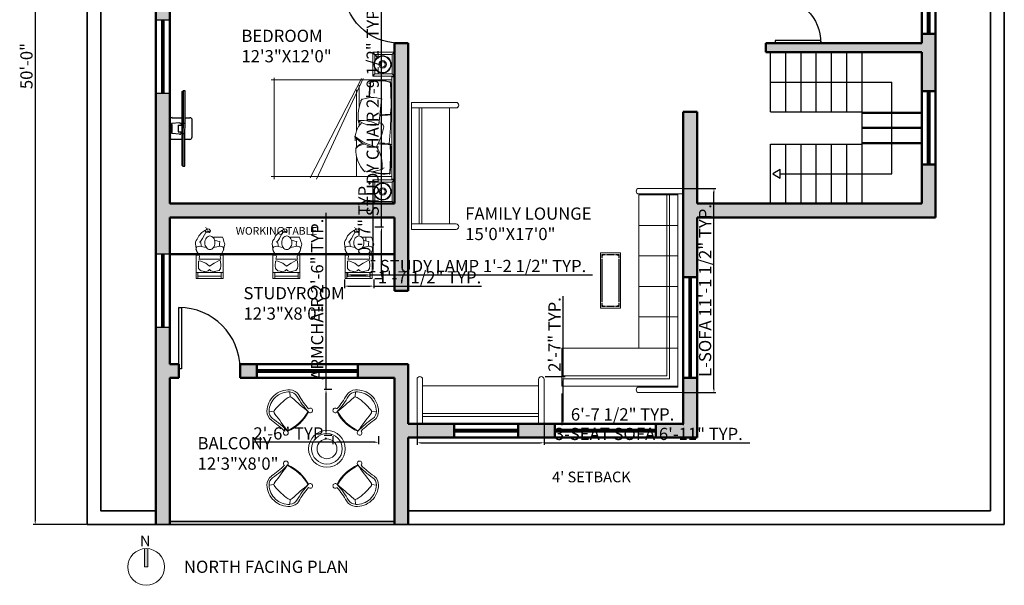
# Model space of a CAD drawing. Units: inches. Extents: x 2442 to 3851, y 589 to 2836.
# Tile 11 of 22: x 3165 to 3809, y 1362 to 1732. Entities that reach past the tile are written whole.
import ezdxf

# ---------------------------------------------------------------- set-up
doc = ezdxf.new("R2010")
doc.units = ezdxf.units.IN
for name, color, linetype, lineweight in [('0.10', 252, 'Continuous', 9), ('0.15', 34, 'Continuous', 15), ('A-ANNO-DIMS', 2, 'Continuous', 18), ('A-ANNO-SYMB', 1, 'Continuous', 18), ('A-ANNO-TEXT', 7, 'Continuous', 18), ('A-AREA-IDEN', 7, 'Continuous', 18), ('A-DOOR', 4, 'Continuous', 25), ('A-FLOR-STRS', 3, 'Continuous', 25), ('A-FURN', 8, 'Continuous', 18), ('A-GLAZ', 1, 'Continuous', 25), ('A-WALL', 7, 'Continuous', 50), ('A-WALL-PATT', 8, 'Continuous', 13), ('C-PROP', 7, 'Continuous', 35)]:
    doc.layers.add(name, color=color, linetype=linetype, lineweight=lineweight)
doc.layers.add('window', color=130, linetype='Continuous')
doc.styles.get("Standard").update_dxf_attribs({"font": 'arial.ttf'})
doc.dimstyles.new('ISO-25', dxfattribs={"dimtxt": 8, "dimasz": 2.5, "dimexe": 1.25, "dimexo": 0.625, "dimtad": 1, "dimlunit": 3, "dimtxsty": 'Standard', "dimcen": 2.5, "dimadec": 0, "dimazin": 0, "dimtfac": 1, "dimtmove": 0, "dimatfit": 3, "dimfxl": 1, "dimarcsym": 0})

# ---------------------------------------------------------------- blocks, each defined once
blk = doc.blocks.new('*U22')
for p, q in [((0, 0), (0, -6)), ((40, 0), (40, -6))]:
    blk.add_line(p, q)
blk.add_lwpolyline([(0, 0), (0, 40), (1.75, 40), (1.75, 0)], close=True)
blk.add_arc((0, 0), 40, 0, 90)
blk = doc.blocks.new('*U23')
for p, q in [((0, 0), (0, -6)), ((36, 0), (36, -6))]:
    blk.add_line(p, q)
blk.add_lwpolyline([(0, 0), (0, 36), (1.75, 36), (1.75, 0)], close=True)
blk.add_arc((0, 0), 36, 0, 90)
blk = doc.blocks.new('*U24')
for p, q in [((0, 0), (0, -6)), ((30, 0), (30, -6))]:
    blk.add_line(p, q)
blk.add_lwpolyline([(0, 0), (0, 30), (1.75, 30), (1.75, 0)], close=True)
blk.add_arc((0, 0), 30, 0, 90)
blk = doc.blocks.new('camita')
at = {"layer": '0.10'}
for p, q in [((-0.85, -0.045), (0.85, -0.045)), ((-0.805, -0.045), (-0.805, -2.048)), ((0.805, -0.045), (0.805, -2.048)), ((-0.827, -0.521), (0.846, -1.293)), ((-0.827, -0.548), (0.824, -1.399)), ((-0.716, -0.585), (-0.355, -0.585)), ((-0.638, -0.63), (0.043, -0.63)), ((-0.114, -0.585), (-0.049, -0.585)), ((0.175, -0.63), (0.318, -0.63)), ((0.474, -0.63), (0.805, -0.63)), ((-0.835, -2), (0.846, -2))]:
    blk.add_line(p, q, dxfattribs=at)
blk.add_lwpolyline([(-0.85, -0.041), (0.85, -0.041), (0.85, 0), (-0.85, 0)], close=True, dxfattribs=at)
for centre, radius, start, end in [((-0.457, -0.236), 0.344, 147.51, 213.8336), ((-0.2, -0.227), 0.586, 163.9263, 197.1409), ((-0.364, -5.846), 5.791, 83.8073, 94.1211), ((-0.51, -1.723), 1.678, 80.1255, 98.6619), ((2.353, -0.053), 2.58, 180.1063, 184.3854), ((-1.544, -0.245), 1.333, 359.9394, 7.5533), ((1.581, -0.289), 1.335, 170.3802, 178.9914), ((-1.44, -0.061), 1.712, 352.9291, 0.3959), ((0.452, -3.067), 3, 83.9026, 93.6759), ((0.486, -1.629), 1.578, 80.1602, 98.06), ((0.029, -0.138), 0.726, 342.5841, 6.0048), ((0.133, -0.17), 0.631, 339.923, 8.7433), ((-0.054, -0.363), 0.454, 159.3026, 206.5026), ((-1.33, -9.675), 9.499, 82.2708, 84.9399), ((0.458, -0.545), 0.584, 151.0456, 184.1497), ((-0.534, -0.339), 0.487, 327.2644, 9.0473), ((-0.007, -0.258), 0.0828, 100.018, 179.736), ((-0.293, -1.438), 1.29, 61.9749, 77.8435), ((-0.199, -0.274), 0.516, 310.7395, 359.0576), ((-0.567, -0.087), 0.906, 321.6953, 346.4626), ((0.627, -0.752), 0.551, 82.9691, 124.6739), ((0.32, -0.394), 0.404, 341.4524, 33.4512), ((-1.867, -14.986), 14.632, 84.6597, 85.7516), ((-0.46, 1.486), 1.909, 260.953, 268.6517), ((-0.2, 0.064), 0.667, 244.7809, 279.0606), ((0.179, -0.272), 0.383, 224.5284, 275.2229), ((0.438, -0.483), 0.19, 193.6849, 236.7035), ((0.571, -0.432), 0.315, 192.9388, 221.9636), ((0.361, -0.133), 0.51, 267.2589, 315.2997)]:
    blk.add_arc(centre, radius, start, end, dxfattribs=at)
blk = doc.blocks.new('VELADOR')
at = {"layer": '0.15'}
for p, q in [((-0.248, 0), (-0.203, -0.045)), ((0.248, 0), (0.202, -0.045)), ((-0.203, -0.405), (-0.248, -0.45)), ((0.248, -0.45), (0.202, -0.405))]:
    blk.add_line(p, q, dxfattribs=at)
blk.add_lwpolyline([(-0.248, 0), (-0.248, -0.45), (0.248, -0.45), (0.248, 0)], close=True, dxfattribs=at)
blk.add_lwpolyline([(0.092, -0.405), (0.202, -0.405), (0.202, -0.045), (-0.203, -0.045), (-0.203, -0.405), (-0.082, -0.405)], dxfattribs=at)
for radius in [0.18, 0.169, 0.0788, 0.0563]:
    blk.add_circle((0.005, -0.247), radius, dxfattribs=at)
blk = doc.blocks.new('TABLE-30A')
at = {"color": 0, "linetype": 'ByBlock'}
for p, q in [((0, 0), (0, 0.55)), ((0, 0.55), (1.5, 0.55)), ((1.5, 0.55), (1.5, 0)), ((0.051, 0.508), (0.042, 0.499)), ((0.042, 0.499), (0.042, 0.478)), ((0.042, 0.478), (0.072, 0.478)), ((0.042, 0.478), (0.042, 0.41)), ((0.042, 0.169), (0.042, 0.381)), ((0.072, 0.508), (0.051, 0.508)), ((0.051, 0.478), (0.051, 0.41)), ((0.051, 0.169), (0.051, 0.381)), ((0.072, 0.478), (0.072, 0.508)), ((0.072, 0.508), (0.14, 0.508)), ((0.072, 0.499), (0.14, 0.499)), ((1.331, 0.508), (0.169, 0.508)), ((1.331, 0.499), (0.169, 0.499)), ((1.428, 0.508), (1.36, 0.508)), ((1.428, 0.499), (1.36, 0.499)), ((1.428, 0.508), (1.428, 0.478)), ((1.449, 0.508), (1.428, 0.508)), ((1.428, 0.478), (1.458, 0.478)), ((1.458, 0.499), (1.449, 0.508)), ((1.449, 0.478), (1.449, 0.41)), ((1.449, 0.381), (1.449, 0.169)), ((1.458, 0.478), (1.458, 0.499)), ((1.458, 0.478), (1.458, 0.41)), ((1.458, 0.381), (1.458, 0.169)), ((1.5, 0), (0, 0)), ((0.042, 0.072), (0.042, 0.14)), ((0.042, 0.072), (0.042, 0.051)), ((0.072, 0.072), (0.042, 0.072)), ((0.042, 0.051), (0.051, 0.042)), ((0.051, 0.072), (0.051, 0.14)), ((0.051, 0.042), (0.072, 0.042)), ((0.072, 0.042), (0.072, 0.072)), ((0.072, 0.051), (0.14, 0.051)), ((0.072, 0.042), (0.14, 0.042)), ((0.169, 0.051), (1.331, 0.051)), ((0.169, 0.042), (1.331, 0.042)), ((1.428, 0.051), (1.36, 0.051)), ((1.428, 0.042), (1.36, 0.042)), ((1.428, 0.072), (1.428, 0.042)), ((1.458, 0.072), (1.428, 0.072)), ((1.428, 0.042), (1.449, 0.042)), ((1.449, 0.072), (1.449, 0.14)), ((1.449, 0.042), (1.458, 0.051)), ((1.458, 0.072), (1.458, 0.14)), ((1.458, 0.051), (1.458, 0.072))]:
    blk.add_line(p, q, dxfattribs=at)
blk = doc.blocks.new('TV')
at = {"color": 0}
for p, q in [((3967.27, 1784.85), (3967.05, 1784.65)), ((3967.76, 1763.68), (3967.54, 1763.86))]:
    blk.add_line(p, q, dxfattribs=at)
at = {"layer": 'window'}
for p, q in [((3967.54, 1763.86), (3967.05, 1784.65)), ((3964.41, 1777.23), (3967.22, 1777.3)), ((3968.01, 1777.32), (3969.36, 1777.35)), ((3966.53, 1775.82), (3964.33, 1775.61)), ((3964.34, 1775.34), (3964.45, 1775.34)), ((3964.34, 1775.31), (3964.43, 1775.32)), ((3966.14, 1775.2), (3967.01, 1775.22)), ((3966.14, 1775.18), (3967.27, 1775.2)), ((3966.14, 1775.18), (3966.14, 1775.2)), ((3966.3, 1773.29), (3966.26, 1775.18)), ((3964.39, 1773.06), (3964.48, 1773.06)), ((3964.39, 1773.04), (3964.5, 1773.04)), ((3966.61, 1772.66), (3964.4, 1772.77)), ((3966.19, 1773.28), (3967.31, 1773.31)), ((3966.19, 1773.26), (3967.05, 1773.28)), ((3966.19, 1773.26), (3966.19, 1773.28)), ((3964.55, 1771.15), (3967.36, 1771.22)), ((3968.15, 1771.24), (3969.5, 1771.27))]:
    blk.add_line(p, q, dxfattribs=at)
for points in [[(3968.33, 1763.69), (3967.83, 1784.86), (3967.27, 1784.85), (3967.76, 1763.68), (3968.33, 1763.69)], [(3963.86, 1771.81), (3963.75, 1776.54)], [(3964.4, 1772.77), (3964.33, 1775.61)], [(3964.48, 1773.06), (3964.43, 1775.32)], [(3964.5, 1773.04), (3964.45, 1775.34)], [(3970.16, 1771.96), (3970.05, 1776.69)]]:
    blk.add_lwpolyline(points, dxfattribs=at)
for points in [[(3966.53, 1775.82, -0.263666), (3966.93, 1775.69), (3967, 1775.57), (3967.01, 1775.22)], [(3966.61, 1772.66, 0.263666), (3967, 1772.81), (3967.06, 1772.93), (3967.05, 1773.28)]]:
    blk.add_lwpolyline(points, format="xyb", dxfattribs=at)
for centre, radius in [((3963.91, 1775.73), 0.0679), ((3963.93, 1775.17), 0.0679), ((3963.94, 1774.6), 0.0679), ((3967.77, 1775.68), 0.0451), ((3963.95, 1774.04), 0.0679), ((3963.97, 1773.48), 0.0679), ((3963.98, 1772.92), 0.0679), ((3963.99, 1772.35), 0.0679), ((3964.01, 1771.79), 0.0679), ((3967.83, 1772.86), 0.0451)]:
    blk.add_circle(centre, radius, dxfattribs=at)
for centre, start, end in [((3964.42, 1776.56), 91.3414, 181.3414), ((3969.38, 1776.67), 1.3414, 91.3414), ((3964.53, 1771.83), 181.3414, 271.3414), ((3969.49, 1771.94), 271.3414, 1.3414)]:
    blk.add_arc(centre, 0.676, start, end, dxfattribs=at)
blk = doc.blocks.new('A$C16EC238A')
for p, q in [((490, 810), (485, 914)), ((148, 493), (45, 507))]:
    blk.add_line(p, q)
for centre, radius, start, end in [((464, 496), 464, 87.0599, 178.502), ((464, 496), 419, 87.0599, 178.502), ((476, 730), 184, 31.9256, 87.0599), ((476, 730), 229, 31.9256, 87.0599), ((2169, 1687), 1715, 209.219, 221.1077), ((1301, -402), 1474, 132.9725, 140.5328), ((1209, -303), 1339, 124.646, 132.9725), ((486, 744), 66, 46.736, 125.0291), ((4628, 5145), 5977, 226.736, 231.1302), ((2169, 1687), 1760, 209.219, 222.7724), ((229, 502), 229, 178.502, 233.6363), ((229, 502), 184, 178.502, 233.6363), ((214, 493), 66, 140.5328, 218.8259), ((-4494, -3296), 5977, 34.4317, 38.8259), ((62, 930), 910, 293.6787, 331.8832), ((62, 930), 925, 293.8563, 331.7056), ((913, 525), 50, 222.7809, 137.6785), ((-856, -1112), 1715, 44.4541, 56.3429), ((-856, -1112), 1760, 42.7895, 56.3429), ((399, 50), 50, 127.8834, 42.7809)]:
    blk.add_arc(centre, radius, start, end)
blk = doc.blocks.new('SOFA-L')
for p, q in [((79.48, 133.62), (50.46, 133.62)), ((79.48, 129.99), (50.46, 129.99)), ((50.46, 129.38), (50.46, 29.02)), ((75.86, 129.38), (50.46, 129.38)), ((75.86, 129.38), (50.46, 129.38)), ((75.86, 3.63), (75.86, 129.99)), ((79.48, 0), (79.48, 133.62)), ((75.86, 29.02), (0, 29.02)), ((0, 4.23), (0, 29.02)), ((75.86, 4.23), (0, 4.23)), ((50.46, 3.63), (75.86, 3.63)), ((50.46, 0), (79.48, 0))]:
    blk.add_line(p, q)
for centre in [(50.46, 131.8), (50.46, 1.81)]:
    blk.add_arc(centre, 1.81, 90, 270)
blk = doc.blocks.new('SOFA-3SEAT')
for p, q in [((0, 29.02), (0, 0)), ((3.63, 0), (3.63, 29.02)), ((79.48, 29.02), (79.48, 0)), ((83.11, 29.02), (83.11, 0)), ((83.11, 0), (0, 0))]:
    blk.add_line(p, q)
for centre in [(1.81, 29.02), (81.3, 29.02)]:
    blk.add_arc(centre, 1.81, 0, 180)
blk = doc.blocks.new('CHAIR-STUDY')
for p, q in [((1.15, 25.77), (2.16, 27.79)), ((2.16, 27.79), (4.26, 29.99)), ((4.75, 26.15), (3.77, 24.72)), ((4.26, 29.99), (6.18, 31.25)), ((5.9, 28.53), (4.75, 26.15)), ((6.88, 29.96), (5.9, 28.53)), ((6.18, 31.25), (6.88, 29.96)), ((6.28, 31), (6.42, 31.35)), ((6.42, 31.35), (7.3, 29.99)), ((7.3, 29.99), (6.81, 29.78)), ((0.69, 17.96), (0, 22.54)), ((0.66, 20.05), (1.01, 20.69)), ((1.01, 20.69), (2.7, 21.06)), ((3.31, 24.09), (2.58, 23.78)), ((2.7, 21.06), (7.03, 20.31)), ((3.77, 24.72), (3.31, 24.09)), ((16.25, 21.06), (11.92, 20.31)), ((17.95, 20.69), (16.25, 21.06)), ((18.3, 20.05), (17.95, 20.69)), ((0.45, 15.23), (0.45, 0)), ((2.33, 15.23), (0.45, 15.23)), ((2.4, 15.12), (0.69, 17.96)), ((2.33, 12.6), (2.59, 13.38)), ((16.63, 12.6), (16.37, 13.38)), ((16.56, 15.12), (18.27, 17.96)), ((18.13, 15.23), (16.63, 15.23)), ((18.13, 0), (18.13, 15.23)), ((16.63, 12.6), (2.33, 12.6)), ((2.33, 12.6), (16.63, 12.6)), ((0.45, 0), (18.13, 0))]:
    blk.add_line(p, q)
at = {"const_width": 0.409}
blk.add_lwpolyline([(9.11, 30.03), (6.61, 33.6)], dxfattribs=at)
for points in [[(6.42, 31.35), (7.08, 31.7), (7.84, 32.37), (9.02, 32.27), (9.83, 31.21), (9.51, 30.11), (9.15, 30.13), (9.15, 30.74), (8.18, 30.77), (7.71, 30.22), (8.96, 29.96)], [(1.15, 25.77), (0.46, 24.74), (0.15, 23.71), (0, 22.89), (0, 22.43)], [(18.27, 17.96), (19.26, 22.38), (18.7, 24.07), (18.13, 26.14), (17.76, 27.08), (16.06, 26.89), (14.37, 26.89), (11.92, 26.89)], [(3.31, 24.09), (3.55, 23.1), (3.8, 21.81), (3.8, 20.89)]]:
    blk.add_lwpolyline(points)
for centre, start, end in [((2.48, 19.04), 150.9331, 210.97654), ((16.48, 19.04), 329.02346, 29.0669), ((0.61, 14.04), 341.55636, 30.97654), ((18.35, 14.04), 149.02346, 198.44364)]:
    blk.add_arc(centre, 2.08, start, end)
blk = doc.blocks.new('STUDY-LAMP')
for p, q in [((0.18, 6.7), (0, 3.72)), ((0.24, 6.78), (0.94, 6.92)), ((0.94, 6.92), (4.89, 5.41)), ((10.35, 5.41), (13.55, 7.11)), ((13.55, 7.11), (14.43, 6.93)), ((14.49, 6.86), (14.68, 3.72)), ((0, 3.72), (0.19, 2.03)), ((0.19, 2.03), (0.72, 1.29)), ((1.8, 0.51), (3.15, 0.09)), ((4.02, 0.02), (5.75, 0.23)), ((4.89, 5.41), (7.34, 3.53)), ((7.12, 1), (7.34, 1.28)), ((7.34, 3.53), (10.35, 5.41)), ((7.56, 1), (7.34, 1.28)), ((10.66, 0.02), (8.93, 0.23)), ((13.55, 0.71), (11.53, 0.09)), ((14.49, 2.03), (13.55, 0.71)), ((14.68, 3.72), (14.49, 2.03))]:
    blk.add_line(p, q)
for centre, radius, start, end in [((0.26, 6.7), 0.0819, 101.30436, 176.63184), ((14.41, 6.85), 0.0819, 3.36816, 78.69563), ((14.41, 6.85), 0.0819, 3.36816, 78.69563), ((2.42, 2.5), 2.08, 215.55138, 252.90541), ((3.76, 2.08), 2.08, 252.90541, 277.12145), ((5.49, 2.3), 2.08, 277.12145, 321.32606), ((9.19, 2.3), 2.08, 218.67394, 262.87855), ((10.92, 2.08), 2.08, 262.87855, 287.09459)]:
    blk.add_arc(centre, radius, start, end)
blk = doc.blocks.new('NORTH-ARROW')
at = {"transparency": 33554687}
h = blk.add_hatch(color=256, dxfattribs=at)
h.dxf.hatch_style = 1
h.paths.add_polyline_path([(13, 12), (11, 12), (11, 23.96, -0.020861), (12, 24, -0.020861), (13, 23.96)])
for p, q in [((11, 24), (11, 12)), ((13, 12), (13, 23.96)), ((11, 12), (13, 12))]:
    blk.add_line(p, q)
blk.add_circle((12, 12), 12)
blk.add_text('N', height=6.9).set_placement((7.98, 25.6))
blk = doc.blocks.new('*D160')
at = {"layer": 'A-ANNO-DIMS', "color": 0, "lineweight": -2, "transparency": 16777216}
for p, q in [((3365.04, 1490.25), (3365.04, 1605.94)), ((3368.91, 1490.25), (3363.79, 1490.25)), ((3365.04, 1462.77), (3365.04, 1487.75)), ((3368.91, 1460.27), (3363.79, 1460.27))]:
    blk.add_line(p, q, dxfattribs=at)
at = {"layer": 'A-ANNO-DIMS', "color": 0, "transparency": 16777216}
for points in [[(3364.62, 1487.75), (3365.46, 1487.75), (3365.04, 1490.25)], [(3364.62, 1462.77), (3365.46, 1462.77), (3365.04, 1460.27)]]:
    blk.add_solid(points, dxfattribs=at)
at = {"layer": 'Defpoints', "color": 0, "transparency": 16777216}
for p in [(3365.04, 1490.25), (3369.54, 1490.25), (3369.54, 1460.27)]:
    blk.add_point(p, dxfattribs=at)
at = {"layer": 'A-ANNO-DIMS', "color": 0, "transparency": 16777216, "insert": (3360.28, 1549.35), "char_height": 8, "attachment_point": 5, "rotation": 90}
blk.add_mtext('ARMCHAIR 2\'-6" TYP.', dxfattribs=at)
blk = doc.blocks.new('*D161')
at = {"layer": 'A-ANNO-DIMS', "color": 0, "lineweight": -2, "transparency": 16777216}
for p, q in [((3369.54, 1459.65), (3369.54, 1454.53)), ((3399.46, 1459.65), (3399.46, 1454.53)), ((3369.54, 1455.78), (3316.89, 1455.78)), ((3396.96, 1455.78), (3372.04, 1455.78))]:
    blk.add_line(p, q, dxfattribs=at)
at = {"layer": 'A-ANNO-DIMS', "color": 0, "transparency": 16777216}
for points in [[(3372.04, 1456.19), (3372.04, 1455.36), (3369.54, 1455.78)], [(3396.96, 1456.19), (3396.96, 1455.36), (3399.46, 1455.78)]]:
    blk.add_solid(points, dxfattribs=at)
at = {"layer": 'Defpoints', "color": 0, "transparency": 16777216}
for p in [(3369.54, 1460.27), (3399.46, 1460.27), (3369.54, 1455.78)]:
    blk.add_point(p, dxfattribs=at)
at = {"layer": 'A-ANNO-DIMS', "color": 0, "transparency": 16777216, "insert": (3341.96, 1460.49), "char_height": 8, "attachment_point": 5}
blk.add_mtext('2\'-6" TYP.', dxfattribs=at)
blk = doc.blocks.new('*D162')
at = {"layer": 'A-ANNO-DIMS', "color": 0, "lineweight": -2, "transparency": 16777216}
for p, q in [((3424.62, 1467.24), (3424.62, 1454.15)), ((3507.73, 1467.24), (3507.73, 1454.15)), ((3427.12, 1455.4), (3505.23, 1455.4)), ((3507.73, 1455.4), (3642.22, 1455.4))]:
    blk.add_line(p, q, dxfattribs=at)
at = {"layer": 'A-ANNO-DIMS', "color": 0, "transparency": 16777216}
for points in [[(3427.12, 1455.81), (3427.12, 1454.98), (3424.62, 1455.4)], [(3505.23, 1455.81), (3505.23, 1454.98), (3507.73, 1455.4)]]:
    blk.add_solid(points, dxfattribs=at)
at = {"layer": 'Defpoints', "color": 0, "transparency": 16777216}
for p in [(3424.62, 1467.86), (3507.73, 1467.86), (3507.73, 1455.4)]:
    blk.add_point(p, dxfattribs=at)
at = {"layer": 'A-ANNO-DIMS', "color": 0, "transparency": 16777216, "insert": (3576.22, 1460.16), "char_height": 8, "attachment_point": 5}
blk.add_mtext('3-SEAT SOFA 6\'-11" TYP.', dxfattribs=at)
blk = doc.blocks.new('*D163')
at = {"layer": 'A-ANNO-DIMS', "color": 0, "lineweight": -2, "transparency": 16777216}
for p, q in [((3520.19, 1498.7), (3520.19, 1551.35)), ((3508.35, 1498.7), (3521.44, 1498.7)), ((3520.19, 1470.36), (3520.19, 1496.2)), ((3508.35, 1467.86), (3521.44, 1467.86))]:
    blk.add_line(p, q, dxfattribs=at)
at = {"layer": 'A-ANNO-DIMS', "color": 0, "transparency": 16777216}
for points in [[(3519.78, 1496.2), (3520.61, 1496.2), (3520.19, 1498.7)], [(3519.78, 1470.36), (3520.61, 1470.36), (3520.19, 1467.86)]]:
    blk.add_solid(points, dxfattribs=at)
at = {"layer": 'Defpoints', "color": 0, "transparency": 16777216}
for p in [(3507.73, 1498.7), (3520.19, 1498.7), (3507.73, 1467.86)]:
    blk.add_point(p, dxfattribs=at)
at = {"layer": 'A-ANNO-DIMS', "color": 0, "transparency": 16777216, "insert": (3515.55, 1526.27), "char_height": 8, "attachment_point": 5, "rotation": 90}
blk.add_mtext('2\'-7" TYP.', dxfattribs=at)
blk = doc.blocks.new('*D164')
at = {"layer": 'A-ANNO-DIMS', "color": 0, "lineweight": -2, "transparency": 16777216}
for p, q in [((3378.99, 1566.84), (3378.99, 1564.02)), ((3393.67, 1566.84), (3393.67, 1564.02)), ((3381.49, 1565.27), (3391.17, 1565.27)), ((3393.67, 1565.27), (3539.31, 1565.27))]:
    blk.add_line(p, q, dxfattribs=at)
at = {"layer": 'A-ANNO-DIMS', "color": 0, "transparency": 16777216}
for points in [[(3381.49, 1565.68), (3381.49, 1564.85), (3378.99, 1565.27)], [(3391.17, 1565.68), (3391.17, 1564.85), (3393.67, 1565.27)]]:
    blk.add_solid(points, dxfattribs=at)
at = {"layer": 'Defpoints', "color": 0, "transparency": 16777216}
for p in [(3378.99, 1567.47), (3393.67, 1567.47), (3393.67, 1565.27)]:
    blk.add_point(p, dxfattribs=at)
at = {"layer": 'A-ANNO-DIMS', "color": 0, "transparency": 16777216, "insert": (3467.74, 1570.03), "char_height": 8, "attachment_point": 5}
blk.add_mtext('STUDY LAMP 1\'-2 1/2" TYP.', dxfattribs=at)
blk = doc.blocks.new('*D165')
at = {"layer": 'A-ANNO-DIMS', "color": 0, "lineweight": -2, "transparency": 16777216}
for p, q in [((3395.87, 1574.59), (3395.87, 1627.11)), ((3394.29, 1574.59), (3397.12, 1574.59)), ((3395.87, 1569.97), (3395.87, 1572.09)), ((3394.29, 1567.47), (3397.12, 1567.47))]:
    blk.add_line(p, q, dxfattribs=at)
at = {"layer": 'A-ANNO-DIMS', "color": 0, "transparency": 16777216}
for points in [[(3395.45, 1572.09), (3396.29, 1572.09), (3395.87, 1574.59)], [(3395.45, 1569.97), (3396.29, 1569.97), (3395.87, 1567.47)]]:
    blk.add_solid(points, dxfattribs=at)
at = {"layer": 'Defpoints', "color": 0, "transparency": 16777216}
for p in [(3393.67, 1574.59), (3395.87, 1574.59), (3393.67, 1567.47)]:
    blk.add_point(p, dxfattribs=at)
at = {"layer": 'A-ANNO-DIMS', "color": 0, "transparency": 16777216, "insert": (3391.16, 1602.1), "char_height": 8, "attachment_point": 5, "rotation": 90}
blk.add_mtext('0\'-7" TYP.', dxfattribs=at)
blk = doc.blocks.new('*D170')
at = {"layer": 'A-ANNO-DIMS', "color": 0, "lineweight": -2, "transparency": 16777216}
for p, q in [((3599.42, 1621.85), (3620.09, 1621.85)), ((3618.84, 1490.73), (3618.84, 1619.35)), ((3599.42, 1488.23), (3620.09, 1488.23))]:
    blk.add_line(p, q, dxfattribs=at)
at = {"layer": 'A-ANNO-DIMS', "color": 0, "transparency": 16777216}
for points in [[(3618.42, 1619.35), (3619.26, 1619.35), (3618.84, 1621.85)], [(3618.42, 1490.73), (3619.26, 1490.73), (3618.84, 1488.23)]]:
    blk.add_solid(points, dxfattribs=at)
at = {"layer": 'Defpoints', "color": 0, "transparency": 16777216}
for p in [(3598.8, 1621.85), (3618.84, 1621.85), (3598.8, 1488.23)]:
    blk.add_point(p, dxfattribs=at)
at = {"layer": 'A-ANNO-DIMS', "color": 0, "transparency": 16777216, "insert": (3614.08, 1555.04), "char_height": 8, "attachment_point": 5, "rotation": 90}
blk.add_mtext('L-SOFA 11\'-1 1/2" TYP.', dxfattribs=at)
blk = doc.blocks.new('*D171')
at = {"layer": 'A-ANNO-DIMS', "color": 0, "lineweight": -2, "transparency": 16777216}
for p, q in [((3519.31, 1487.6), (3519.31, 1466.93)), ((3598.8, 1487.6), (3598.8, 1466.93)), ((3521.81, 1468.18), (3596.3, 1468.18))]:
    blk.add_line(p, q, dxfattribs=at)
at = {"layer": 'A-ANNO-DIMS', "color": 0, "transparency": 16777216}
for points in [[(3521.81, 1468.6), (3521.81, 1467.77), (3519.31, 1468.18)], [(3596.3, 1468.6), (3596.3, 1467.77), (3598.8, 1468.18)]]:
    blk.add_solid(points, dxfattribs=at)
at = {"layer": 'Defpoints', "color": 0, "transparency": 16777216}
for p in [(3519.31, 1488.23), (3598.8, 1488.23), (3598.8, 1468.18)]:
    blk.add_point(p, dxfattribs=at)
at = {"layer": 'A-ANNO-DIMS', "color": 0, "transparency": 16777216, "insert": (3559.06, 1472.95), "char_height": 8, "attachment_point": 5}
blk.add_mtext('6\'-7 1/2" TYP.', dxfattribs=at)
blk = doc.blocks.new('*D172')
at = {"layer": 'A-ANNO-DIMS', "color": 0, "lineweight": -2, "transparency": 16777216}
for p, q in [((3401.36, 1596.65), (3401.36, 1746.62)), ((3396.93, 1596.65), (3402.61, 1596.65)), ((3401.36, 1565.43), (3401.36, 1594.15)), ((3396.93, 1562.93), (3402.61, 1562.93))]:
    blk.add_line(p, q, dxfattribs=at)
at = {"layer": 'A-ANNO-DIMS', "color": 0, "transparency": 16777216}
for points in [[(3400.94, 1594.15), (3401.78, 1594.15), (3401.36, 1596.65)], [(3400.94, 1565.43), (3401.78, 1565.43), (3401.36, 1562.93)]]:
    blk.add_solid(points, dxfattribs=at)
at = {"layer": 'Defpoints', "color": 0, "transparency": 16777216}
for p in [(3396.3, 1596.65), (3401.36, 1596.65), (3396.3, 1562.93)]:
    blk.add_point(p, dxfattribs=at)
at = {"layer": 'A-ANNO-DIMS', "color": 0, "transparency": 16777216, "insert": (3396.6, 1672.89), "char_height": 8, "attachment_point": 5, "rotation": 90}
blk.add_mtext('STUDY CHAIR 2\'-9 1/2" TYP.', dxfattribs=at)
blk = doc.blocks.new('*D173')
at = {"layer": 'A-ANNO-DIMS', "color": 0, "lineweight": -2, "transparency": 16777216}
for p, q in [((3377.04, 1562.31), (3377.04, 1556.63)), ((3396.3, 1562.31), (3396.3, 1556.63)), ((3379.54, 1557.88), (3393.8, 1557.88)), ((3396.3, 1557.88), (3466.71, 1557.88))]:
    blk.add_line(p, q, dxfattribs=at)
at = {"layer": 'A-ANNO-DIMS', "color": 0, "transparency": 16777216}
for points in [[(3379.54, 1558.29), (3379.54, 1557.46), (3377.04, 1557.88)], [(3393.8, 1558.29), (3393.8, 1557.46), (3396.3, 1557.88)]]:
    blk.add_solid(points, dxfattribs=at)
at = {"layer": 'Defpoints', "color": 0, "transparency": 16777216}
for p in [(3377.04, 1562.93), (3396.3, 1562.93), (3396.3, 1557.88)]:
    blk.add_point(p, dxfattribs=at)
at = {"layer": 'A-ANNO-DIMS', "color": 0, "transparency": 16777216, "insert": (3432.76, 1562.64), "char_height": 8, "attachment_point": 5}
blk.add_mtext('1\'-7 1/2" TYP.', dxfattribs=at)
blk = doc.blocks.new('*D257')
at = {"layer": 'A-ANNO-DIMS', "color": 0, "lineweight": -2, "transparency": 16777216}
for p, q in [((3208.17, 2001.86), (3173.55, 2001.86)), ((3174.8, 1999.36), (3174.8, 1404.36)), ((3208.17, 1401.86), (3173.55, 1401.86))]:
    blk.add_line(p, q, dxfattribs=at)
at = {"layer": 'A-ANNO-DIMS', "color": 0, "transparency": 16777216}
for points in [[(3174.38, 1999.36), (3175.21, 1999.36), (3174.8, 2001.86)], [(3174.38, 1404.36), (3175.21, 1404.36), (3174.8, 1401.86)]]:
    blk.add_solid(points, dxfattribs=at)
at = {"layer": 'Defpoints', "color": 0, "transparency": 16777216}
for p in [(3208.8, 2001.86), (3174.8, 1401.86), (3208.8, 1401.86)]:
    blk.add_point(p, dxfattribs=at)
at = {"layer": 'A-ANNO-DIMS', "color": 0, "transparency": 16777216, "insert": (3170.09, 1701.86), "char_height": 8, "attachment_point": 5, "rotation": 90}
blk.add_mtext('50\'-0"', dxfattribs=at)

msp = doc.modelspace()

# ---------------------------------------------------------------- hatches: boundary and pattern name
at = {"layer": 'A-WALL-PATT'}
h = msp.add_hatch(color=256, dxfattribs=at)
h.dxf.hatch_style = 1
h.paths.add_polyline_path([(3262.798, 1497.864), (3268.798, 1497.864), (3268.798, 1503.864), (3268.798, 1506.864), (3262.798, 1506.864), (3262.798, 1530.864), (3253.798, 1530.864), (3253.798, 1401.864), (3262.798, 1401.864)])
h.paths.add_polyline_path([(3418.798, 1506.864), (3385.798, 1506.864), (3385.798, 1497.864), (3409.798, 1497.864), (3409.798, 1401.864), (3418.798, 1401.864), (3418.798, 1458.864), (3448.798, 1458.864), (3448.798, 1467.864), (3424.616, 1467.864), (3418.798, 1467.864)])
h.paths.add_polyline_path([(3319.798, 1506.864), (3308.798, 1506.864), (3308.798, 1497.864), (3319.798, 1497.864)])
h.paths.add_polyline_path([(3514.798, 1467.864), (3490.798, 1467.864), (3490.798, 1458.864), (3514.798, 1458.864)])
h.paths.add_polyline_path([(3607.798, 1497.864), (3598.798, 1497.864), (3598.798, 1488.228), (3598.798, 1467.864), (3580.798, 1467.864), (3580.798, 1458.864), (3607.798, 1458.864)])
h.paths.add_polyline_path([(3418.798, 1716.864), (3409.798, 1716.864), (3409.798, 1611.864), (3262.798, 1611.864), (3262.798, 1683.864), (3253.798, 1683.864), (3253.798, 1578.864), (3262.798, 1578.864), (3262.798, 1602.864), (3409.798, 1602.864), (3409.798, 1554.864), (3418.798, 1554.864)])
h.paths.add_polyline_path([(3418.798, 1767.864), (3406.798, 1767.864), (3406.798, 1764.864), (3262.798, 1764.864), (3262.798, 1820.364), (3253.798, 1820.364), (3253.798, 1731.864), (3262.798, 1731.864), (3262.798, 1755.864), (3409.798, 1755.864), (3409.798, 1752.864), (3412.798, 1752.864), (3418.798, 1752.864)])
h.paths.add_polyline_path([(3355.798, 1932.864), (3253.798, 1932.864), (3253.798, 1868.364), (3262.798, 1868.364), (3262.798, 1907.939), (3262.798, 1923.864), (3276.934, 1923.864), (3355.798, 1923.864), (3355.798, 1929.864)])
h.paths.add_polyline_path([(3415.798, 1992.864), (3406.798, 1992.864), (3406.798, 1932.864), (3385.798, 1932.864), (3385.798, 1923.864), (3406.798, 1923.864), (3406.798, 1803.864), (3415.798, 1803.864), (3415.798, 1818.864), (3514.798, 1818.864), (3514.798, 1827.864), (3415.798, 1827.864), (3415.798, 1947.864), (3445.798, 1947.864), (3445.798, 1956.864), (3415.798, 1956.864)])
h.paths.add_polyline_path([(3565.798, 1956.864), (3511.798, 1956.864), (3511.798, 1947.864), (3514.798, 1947.864), (3553.798, 1947.864), (3553.798, 1827.864), (3550.798, 1827.864), (3550.798, 1824.864), (3550.798, 1818.864), (3553.798, 1818.864), (3553.798, 1764.864), (3565.798, 1764.864), (3565.798, 1770.864), (3565.798, 1773.864), (3562.798, 1773.864), (3562.798, 1947.864), (3565.798, 1947.864)])
h.paths.add_polyline_path([(3682.798, 1956.864), (3613.798, 1956.864), (3613.798, 1947.864), (3682.798, 1947.864)])
h.paths.add_polyline_path([(3763.798, 1956.864), (3730.798, 1956.864), (3730.798, 1947.864), (3754.798, 1947.864), (3754.798, 1875.864), (3763.798, 1875.864)])
h.paths.add_polyline_path([(3763.798, 1827.864), (3661.798, 1827.864), (3661.798, 1821.864), (3754.798, 1821.864), (3754.798, 1815.864), (3763.798, 1815.864)])
h.paths.add_polyline_path([(3763.798, 1779.864), (3754.798, 1779.864), (3754.798, 1773.864), (3707.032, 1773.864, -0.0790467), (3706.561, 1773.864), (3676.798, 1773.864), (3676.798, 1791.864), (3670.798, 1791.864), (3670.798, 1773.864), (3610.798, 1773.864), (3610.798, 1821.864), (3631.798, 1821.864), (3631.798, 1827.864), (3604.798, 1827.864), (3604.798, 1773.864), (3601.798, 1773.864), (3601.798, 1764.864), (3652.798, 1764.864), (3652.798, 1746.864), (3658.798, 1746.864), (3658.798, 1764.864), (3671.259, 1764.864), (3754.798, 1764.864), (3754.798, 1758.864), (3763.798, 1758.864)])
h.paths.add_polyline_path([(3763.798, 1722.864), (3754.798, 1722.864), (3754.798, 1716.864), (3652.798, 1716.864), (3652.798, 1710.864), (3754.798, 1710.864), (3754.798, 1685.364), (3763.798, 1685.364)])
h.paths.add_polyline_path([(3607.798, 1671.864), (3598.798, 1671.864), (3598.798, 1563.864), (3607.798, 1563.864), (3607.798, 1602.864), (3763.798, 1602.864), (3763.798, 1637.364), (3754.798, 1637.364), (3754.798, 1611.864), (3607.798, 1611.864)])

# ---------------------------------------------------------------- linework, layer by layer
at = {"layer": 'A-FLOR-STRS'}
for p, q in [((3655.798, 1671.864), (3655.798, 1710.864)), ((3665.798, 1671.864), (3665.798, 1710.864)), ((3675.798, 1671.864), (3675.798, 1710.864)), ((3685.798, 1671.864), (3685.798, 1710.864)), ((3695.798, 1671.864), (3695.798, 1710.864)), ((3705.798, 1671.864), (3705.798, 1710.864)), ((3715.798, 1650.864), (3715.798, 1710.864)), ((3655.798, 1691.364), (3735.298, 1691.364)), ((3735.298, 1631.364), (3735.298, 1691.364)), ((3655.798, 1671.864), (3715.798, 1671.864)), ((3655.798, 1650.864), (3715.798, 1650.864)), ((3662.255, 1631.364), (3735.298, 1631.364))]:
    msp.add_line(p, q, dxfattribs=at)
at = {"layer": 'A-FLOR-STRS', "ltscale": 0.5}
for p, q in [((3655.798, 1611.864), (3655.798, 1650.864)), ((3665.798, 1611.864), (3665.798, 1650.864)), ((3675.798, 1611.864), (3675.798, 1650.864)), ((3685.798, 1611.864), (3685.798, 1650.864)), ((3695.798, 1611.864), (3695.798, 1650.864)), ((3705.798, 1611.864), (3705.798, 1650.864)), ((3715.798, 1611.864), (3715.798, 1650.864))]:
    msp.add_line(p, q, dxfattribs=at)
at = {"layer": 'A-FLOR-STRS'}
msp.add_lwpolyline([(3657.412, 1631.364), (3662.255, 1628.568), (3662.255, 1634.16)], close=True, dxfattribs=at)
at = {"layer": 'A-FURN'}
for p, q in [((3425.908, 1598.632), (3425.908, 1674.488)), ((3427.721, 1598.632), (3427.721, 1674.488)), ((3445.86, 1674.488), (3445.86, 1598.632)), ((3587.915, 1499.111), (3587.915, 1617.612)), ((3589.728, 1497.297), (3589.728, 1617.612)), ((3595.17, 1597.66), (3569.776, 1597.66)), ((3281.733, 1590.726), (3283.829, 1592.926)), ((3283.829, 1592.926), (3285.75, 1594.183)), ((3285.471, 1591.459), (3284.319, 1589.084)), ((3286.449, 1592.891), (3285.471, 1591.459)), ((3285.75, 1594.183), (3286.449, 1592.891)), ((3285.855, 1593.939), (3285.995, 1594.288)), ((3285.995, 1594.288), (3286.869, 1592.926)), ((3286.869, 1592.926), (3286.38, 1592.716)), ((3280.263, 1580.897), (3279.574, 1585.47)), ((3280.72, 1588.701), (3281.733, 1590.726)), ((3282.887, 1587.024), (3282.153, 1586.71)), ((3283.341, 1587.652), (3282.887, 1587.024)), ((3284.319, 1589.084), (3283.341, 1587.652)), ((3280.229, 1582.982), (3280.584, 1583.622)), ((3281.972, 1578.05), (3280.263, 1580.897)), ((3280.584, 1583.622), (3282.278, 1583.998)), ((3282.278, 1583.998), (3286.606, 1583.246)), ((3295.826, 1583.998), (3291.498, 1583.246)), ((3297.52, 1583.622), (3295.826, 1583.998)), ((3296.132, 1578.05), (3297.841, 1580.897)), ((3297.875, 1582.982), (3297.52, 1583.622)), ((3280.02, 1578.168), (3280.02, 1562.934)), ((3281.902, 1578.168), (3280.02, 1578.168)), ((3281.902, 1575.535), (3282.163, 1576.318)), ((3296.202, 1575.535), (3281.902, 1575.535)), ((3281.902, 1575.535), (3296.202, 1575.535)), ((3296.202, 1575.535), (3295.941, 1576.318)), ((3297.708, 1578.168), (3296.202, 1578.168)), ((3297.708, 1562.934), (3297.708, 1578.168)), ((3595.17, 1577.709), (3569.776, 1577.709)), ((3280.02, 1566.883), (3297.708, 1566.883)), ((3281.173, 1566.883), (3281.173, 1562.934)), ((3296.496, 1566.883), (3296.496, 1562.934)), ((3330.314, 1566.883), (3348.002, 1566.883)), ((3331.467, 1566.883), (3331.467, 1562.934)), ((3346.79, 1566.883), (3346.79, 1562.934)), ((3377.487, 1566.883), (3395.175, 1566.883)), ((3378.64, 1566.883), (3378.64, 1562.934)), ((3393.963, 1566.883), (3393.963, 1562.934)), ((3280.02, 1562.934), (3297.708, 1562.934)), ((3281.173, 1564.439), (3296.496, 1564.439)), ((3331.467, 1564.439), (3346.79, 1564.439)), ((3378.64, 1564.439), (3393.963, 1564.439)), ((3595.17, 1557.758), (3569.776, 1557.758)), ((3595.17, 1537.806), (3569.776, 1537.806)), ((3519.315, 1499.111), (3587.915, 1499.111)), ((3519.315, 1497.297), (3589.728, 1497.297)), ((3504.099, 1492.651), (3428.244, 1492.651)), ((3428.244, 1474.513), (3504.099, 1474.513)), ((3428.244, 1472.699), (3504.099, 1472.699))]:
    msp.add_line(p, q, dxfattribs=at)
at = {"layer": 'A-FURN', "const_width": 0.409}
msp.add_lwpolyline([(3288.681, 1592.96), (3286.187, 1596.531)], dxfattribs=at)
at = {"layer": 'A-FURN'}
for points in [[(3285.995, 1594.288), (3286.652, 1594.629), (3287.413, 1595.305), (3288.596, 1595.199), (3289.399, 1594.143), (3289.083, 1593.044), (3288.723, 1593.066), (3288.723, 1593.678), (3287.751, 1593.7), (3287.286, 1593.15), (3288.533, 1592.897)], [(3280.72, 1588.701), (3280.036, 1587.674), (3279.728, 1586.647), (3279.574, 1585.826), (3279.574, 1585.363)], [(3282.887, 1587.024), (3283.119, 1586.031), (3283.376, 1584.747), (3283.376, 1583.823)], [(3297.841, 1580.897), (3298.837, 1585.315), (3298.272, 1587.007), (3297.708, 1589.076), (3297.331, 1590.017), (3295.638, 1589.828), (3293.944, 1589.828), (3291.498, 1589.828)], [(3292.063, 1587.948), (3294.321, 1587.384), (3295.638, 1587.195), (3295.262, 1585.315), (3295.45, 1583.81)], [(3342.357, 1587.948), (3344.615, 1587.384), (3345.932, 1587.195), (3345.555, 1585.315), (3345.744, 1583.81)], [(3389.53, 1587.948), (3391.788, 1587.384), (3393.105, 1587.195), (3392.729, 1585.315), (3392.917, 1583.81)]]:
    msp.add_lwpolyline(points, dxfattribs=at)
for points in [[(3285.784, 1586.254, 0.0740504), (3286.046, 1584.492, 0.0848007), (3286.745, 1583.099, 0.1063356), (3287.864, 1582.108, 0.1289555), (3289.064, 1581.793, 0.1289555), (3290.263, 1582.108, 0.1063356), (3291.383, 1583.099, 0.0848007), (3292.082, 1584.492, 0.0740504), (3292.344, 1586.254, 0.0740504), (3292.082, 1588.015, 0.0848007), (3291.383, 1589.408, 0.1063356), (3290.263, 1590.399, 0.1289555), (3289.064, 1590.714, 0.1289555), (3287.864, 1590.399, 0.1063356), (3286.745, 1589.408, 0.0848007), (3286.046, 1588.015, 0.0740504)], [(3336.078, 1586.254, 0.0740504), (3336.34, 1584.492, 0.0848007), (3337.039, 1583.099, 0.1063356), (3338.158, 1582.108, 0.1289555), (3339.358, 1581.793, 0.1289555), (3340.557, 1582.108, 0.1063356), (3341.677, 1583.099, 0.0848007), (3342.376, 1584.492, 0.0740504), (3342.638, 1586.254, 0.0740504), (3342.376, 1588.015, 0.0848007), (3341.677, 1589.408, 0.1063356), (3340.557, 1590.399, 0.1289555), (3339.358, 1590.714, 0.1289555), (3338.158, 1590.399, 0.1063356), (3337.039, 1589.408, 0.0848007), (3336.34, 1588.015, 0.0740504)], [(3383.251, 1586.254, 0.0740504), (3383.514, 1584.492, 0.0848007), (3384.212, 1583.099, 0.1063356), (3385.332, 1582.108, 0.1289555), (3386.531, 1581.793, 0.1289555), (3387.731, 1582.108, 0.1063356), (3388.851, 1583.099, 0.0848007), (3389.549, 1584.492, 0.0740504), (3389.811, 1586.254, 0.0740504), (3389.549, 1588.015, 0.0848007), (3388.851, 1589.408, 0.1063356), (3387.731, 1590.399, 0.1289555), (3386.531, 1590.714, 0.1289555), (3385.332, 1590.399, 0.1063356), (3384.212, 1589.408, 0.0848007), (3383.514, 1588.015, 0.0740504)]]:
    msp.add_lwpolyline(points, format="xyb", close=True, dxfattribs=at)
for radius in [12, 10, 6.496]:
    msp.add_circle((3365.649, 1451.467), radius, dxfattribs=at)
for centre, start, end in [((3282.051, 1581.969), 150.933101, 210.976536), ((3296.053, 1581.969), 329.023464, 29.066899), ((3280.185, 1576.977), 341.55636, 30.976536), ((3297.919, 1576.977), 149.023464, 198.44364)]:
    msp.add_arc(centre, 2.084, start, end, dxfattribs=at)
at = {"layer": 'A-GLAZ'}
for p, q in [((3262.798, 1731.864), (3253.798, 1731.864)), ((3262.798, 1683.864), (3253.798, 1683.864)), ((3262.798, 1578.864), (3253.798, 1578.864)), ((3262.798, 1530.864), (3253.798, 1530.864))]:
    msp.add_line(p, q, dxfattribs=at)
at = {"layer": 'A-WALL'}
for p, q in [((3253.798, 1992.864), (3253.798, 1401.864)), ((3763.798, 1602.864), (3763.798, 1956.864)), ((3754.798, 1716.864), (3754.798, 1764.864)), ((3758.798, 1722.864), (3758.798, 1758.864)), ((3759.798, 1722.864), (3759.798, 1758.864)), ((3262.798, 1755.864), (3262.798, 1611.864)), ((3257.798, 1731.864), (3257.798, 1683.864)), ((3258.798, 1731.864), (3258.798, 1683.864)), ((3754.798, 1722.864), (3763.798, 1722.864)), ((3409.798, 1611.864), (3409.798, 1716.864)), ((3409.798, 1716.864), (3418.798, 1716.864)), ((3418.798, 1554.864), (3418.798, 1716.864)), ((3652.798, 1710.864), (3652.798, 1716.864)), ((3652.798, 1716.864), (3754.798, 1716.864)), ((3652.798, 1710.864), (3754.798, 1710.864)), ((3754.798, 1611.864), (3754.798, 1710.864)), ((3754.798, 1685.364), (3763.798, 1685.364)), ((3758.798, 1637.364), (3758.798, 1685.364)), ((3759.798, 1637.364), (3759.798, 1685.364)), ((3598.798, 1671.864), (3607.798, 1671.864)), ((3598.798, 1467.864), (3598.798, 1671.864)), ((3607.798, 1611.864), (3607.798, 1671.864)), ((3715.798, 1671.364), (3754.798, 1671.364)), ((3715.798, 1661.364), (3754.798, 1661.364)), ((3715.798, 1651.364), (3754.798, 1651.364)), ((3754.798, 1637.364), (3763.798, 1637.364)), ((3262.798, 1611.864), (3409.798, 1611.864)), ((3607.798, 1611.864), (3754.798, 1611.864)), ((3262.798, 1602.864), (3262.798, 1506.864)), ((3262.798, 1602.864), (3409.798, 1602.864)), ((3409.798, 1554.864), (3409.798, 1602.864)), ((3607.798, 1458.864), (3607.798, 1602.864)), ((3607.798, 1602.864), (3763.798, 1602.864)), ((3257.798, 1578.864), (3257.798, 1530.864)), ((3258.798, 1578.864), (3258.798, 1530.864)), ((3262.798, 1578.864), (3409.798, 1578.864)), ((3598.798, 1563.864), (3607.798, 1563.864)), ((3602.798, 1497.864), (3602.798, 1563.864)), ((3603.798, 1497.864), (3603.798, 1563.864)), ((3409.798, 1554.864), (3418.798, 1554.864)), ((3262.798, 1506.864), (3268.798, 1506.864)), ((3268.798, 1506.864), (3268.798, 1497.864)), ((3308.798, 1506.864), (3308.798, 1497.864)), ((3308.798, 1506.864), (3418.798, 1506.864)), ((3319.798, 1497.864), (3319.798, 1506.864)), ((3319.798, 1502.864), (3385.798, 1502.864)), ((3319.798, 1501.864), (3385.798, 1501.864)), ((3385.798, 1497.864), (3385.798, 1506.864)), ((3418.798, 1467.864), (3418.798, 1506.864)), ((3262.798, 1497.864), (3262.798, 1401.864)), ((3262.798, 1497.864), (3268.798, 1497.864)), ((3308.798, 1497.864), (3409.798, 1497.864)), ((3409.798, 1401.864), (3409.798, 1497.864)), ((3598.798, 1497.864), (3607.798, 1497.864)), ((3418.798, 1467.864), (3598.798, 1467.864)), ((3448.798, 1458.864), (3448.798, 1467.864)), ((3448.798, 1463.864), (3490.798, 1463.864)), ((3448.798, 1462.864), (3490.798, 1462.864)), ((3490.798, 1458.864), (3490.798, 1467.864)), ((3514.798, 1458.864), (3514.798, 1467.864)), ((3514.798, 1463.864), (3580.798, 1463.864)), ((3514.798, 1462.864), (3580.798, 1462.864)), ((3580.798, 1458.864), (3580.798, 1467.864)), ((3418.798, 1458.864), (3607.798, 1458.864)), ((3418.798, 1401.864), (3418.798, 1458.864))]:
    msp.add_line(p, q, dxfattribs=at)
at = {"layer": 'C-PROP'}
for points in [[(3808.798, 1401.864), (3808.798, 2001.864), (3208.798, 2001.864), (3208.798, 1401.864), (3808.798, 1401.864)], [(3799.798, 1410.864), (3799.798, 1992.864), (3217.798, 1992.864), (3217.798, 1410.864), (3253.798, 1410.864)], [(3418.798, 1410.864), (3799.798, 1410.864)], [(3262.798, 1403.864), (3409.798, 1403.864)]]:
    msp.add_lwpolyline(points, dxfattribs=at)

# ---------------------------------------------------------------- block references
at = {"layer": 'A-ANNO-SYMB'}
msp.add_blockref('NORTH-ARROW', (3235.387, 1362.181), dxfattribs=at)
at = {"layer": 'A-DOOR', "xscale": -1}
for name, p, rotation in [('*U23', (3412.798, 1752.864), 90), ('*U24', (3658.798, 1716.864), 270)]:
    msp.add_blockref(name, p, dxfattribs=dict(at, rotation=rotation))
at = {"layer": 'A-DOOR'}
msp.add_blockref('*U22', (3268.798, 1503.864), dxfattribs=at)
at = {"layer": 'A-FURN'}
for name, p, xscale, yscale, zscale, rotation in [('VELADOR', (3409.798, 1703.089), 31.41542173157097, 31.41542173157097, 31.41542173157097, 270), ('camita', (3409.798, 1661.257), 39.375, 39.375, 39.375, 270), ('TV', (-6064.233, -2232.164), 2.327319231123021, 2.327319231123021, 2.327319231123021, 358.5430845181613), ('VELADOR', (3409.798, 1619.639), -31.41542173157097, 31.41542173157097, 31.41542173157097, 269.9999999999999), ('TABLE-30A', (3544.517, 1543.504), -24.08863485716172, 24.08863485716172, 24.08863485716172, 270), ('A$C16EC238A', (3326.412, 1443.489), -0.031001591544, 0.031001591544, 0.031001591544, 180), ('A$C16EC238A', (3399.4, 1443.489), 0.031001591544, 0.031001591544, 0.031001591544, 180)]:
    msp.add_blockref(name, p, dxfattribs=dict(at, xscale=xscale, yscale=yscale, zscale=zscale, rotation=rotation))
at = {"layer": 'A-FURN', "rotation": 270.0000000000016}
msp.add_blockref('SOFA-3SEAT', (3421.073, 1678.115), dxfattribs=at)
at = {"layer": 'A-FURN'}
for name, p in [('SOFA-L', (3519.315, 1488.228)), ('CHAIR-STUDY', (3329.867, 1562.934)), ('CHAIR-STUDY', (3377.041, 1562.934)), ('STUDY-LAMP', (3281.525, 1567.487)), ('STUDY-LAMP', (3331.819, 1567.487)), ('STUDY-LAMP', (3378.992, 1567.487)), ('SOFA-3SEAT', (3424.616, 1467.864))]:
    msp.add_blockref(name, p, dxfattribs=at)
at = {"layer": 'A-FURN', "yscale": 0.031001591544, "zscale": 0.031001591544}
for p, xscale in [((3326.412, 1460.322), 0.031001591544), ((3399.4, 1460.322), -0.031001591544)]:
    msp.add_blockref('A$C16EC238A', p, dxfattribs=dict(at, xscale=xscale))

# ---------------------------------------------------------------- texts
at = {"layer": 'A-ANNO-TEXT', "attachment_point": 1}
for s, width, insert, char_height in [('{\\fTimes New Roman|b0|i0|c0|p18;WORKING TABLE}', 110.76054, (3306.015, 1596.554), 5), ("{\\fTimes New Roman|b0|i0|c0|p18;4' SETBACK}", 79.56037, (3512.937, 1436.558), 7), ('{\\fTimes New Roman|b0|i0|c0|p18;NORTH FACING PLAN}', 196.26071, (3272.08, 1378.304), 8)]:
    msp.add_mtext_dynamic_manual_height_columns(s, width=width, gutter_width=12.5, heights=[0], dxfattribs=dict(at, insert=insert, char_height=char_height))
at = {"layer": 'A-AREA-IDEN', "char_height": 8, "attachment_point": 1}
for s, insert in [('{\\fTimes New Roman|b0|i0|c0|p18;BEDROOM\\P12\'3"X12\'0"}', (3309.722, 1725.631)), ('{\\fTimes New Roman|b0|i0|c0|p18;FAMILY LOUNGE\\P15\'0"X17\'0"}', (3456.145, 1609.338)), ('{\\fTimes New Roman|b0|i0|c0|p18;STUDYROOM\\P12\'3"X8\'0"}', (3311.046, 1557.278)), ('{\\fTimes New Roman|b0|i0|c0|p18;BALCONY\\P12\'3"X8\'0"}', (3280.997, 1459.121))]:
    msp.add_mtext_dynamic_manual_height_columns(s, width=110.76054, gutter_width=12.5, heights=[0], dxfattribs=dict(at, insert=insert))

# ---------------------------------------------------------------- dimensions: what is measured, and where the dimension line sits
at = {"layer": 'A-ANNO-DIMS'}
dim = msp.add_linear_dim(base=(3174.798, 1401.864), p1=(3208.798, 2001.864), p2=(3208.798, 1401.864), angle=90, dimstyle='ISO-25', override={"dimdec": 1, "dimlfac": 1, "dimrnd": 0, "dimzin": 1, "dimdsep": 46, "dimlunit": 4, "dimfrac": 2}, dxfattribs=at)
dim.commit()
dim.dimension.update_dxf_attribs({"geometry": '*D257', "text_midpoint": (3170.088, 1701.864)})
for base, p1, p2, angle, text, picture, middle in [((3401.361, 1596.648), (3396.304, 1562.934), (3396.304, 1596.648), 90, 'STUDY CHAIR <> TYP.', '*D172', (3396.6, 1672.886)), ((3395.871, 1574.595), (3393.67, 1567.467), (3393.67, 1574.595), 90, '<> TYP.', '*D165', (3391.162, 1602.101)), ((3618.84, 1621.846), (3598.798, 1488.228), (3598.798, 1621.846), 90, 'L-SOFA <> TYP.', '*D170', (3614.076, 1555.037)), ((3365.039, 1490.255), (3369.536, 1460.274), (3369.536, 1490.255), 90, 'ARMCHAIR <> TYP.', '*D160', (3360.277, 1549.35)), ((3520.193, 1498.699), (3507.727, 1467.864), (3507.727, 1498.699), 90, '<> TYP.', '*D163', (3515.549, 1526.274)), ((3369.536, 1455.777), (3399.461, 1460.274), (3369.536, 1460.274), 180, '<> TYP.', '*D161', (3341.96, 1460.487))]:
    dim = msp.add_linear_dim(base=base, p1=p1, p2=p2, angle=angle, text=text, dimstyle='ISO-25', override={"dimdec": 1, "dimrnd": 0, "dimzin": 1, "dimlunit": 4, "dimfrac": 2}, dxfattribs=at)
    dim.commit()
    dim.dimension.update_dxf_attribs({"geometry": picture, "text_midpoint": middle})
for base, p1, p2, text, picture, middle in [((3393.67, 1565.265), (3378.993, 1567.467), (3393.67, 1567.467), 'STUDY LAMP <> TYP.', '*D164', (3467.739, 1570.026)), ((3396.304, 1557.877), (3377.041, 1562.934), (3396.304, 1562.934), '<> TYP.', '*D173', (3432.755, 1562.638)), ((3598.798, 1468.185), (3519.315, 1488.228), (3598.798, 1488.228), '<> TYP.', '*D171', (3559.056, 1472.946)), ((3507.727, 1455.397), (3424.616, 1467.864), (3507.727, 1467.864), '3-SEAT SOFA <> TYP.', '*D162', (3576.221, 1460.164))]:
    dim = msp.add_linear_dim(base=base, p1=p1, p2=p2, text=text, dimstyle='ISO-25', override={"dimdec": 1, "dimrnd": 0, "dimzin": 1, "dimlunit": 4, "dimfrac": 2}, dxfattribs=at)
    dim.commit()
    dim.dimension.update_dxf_attribs({"geometry": picture, "text_midpoint": middle})

doc.saveas('drawing.dxf')
